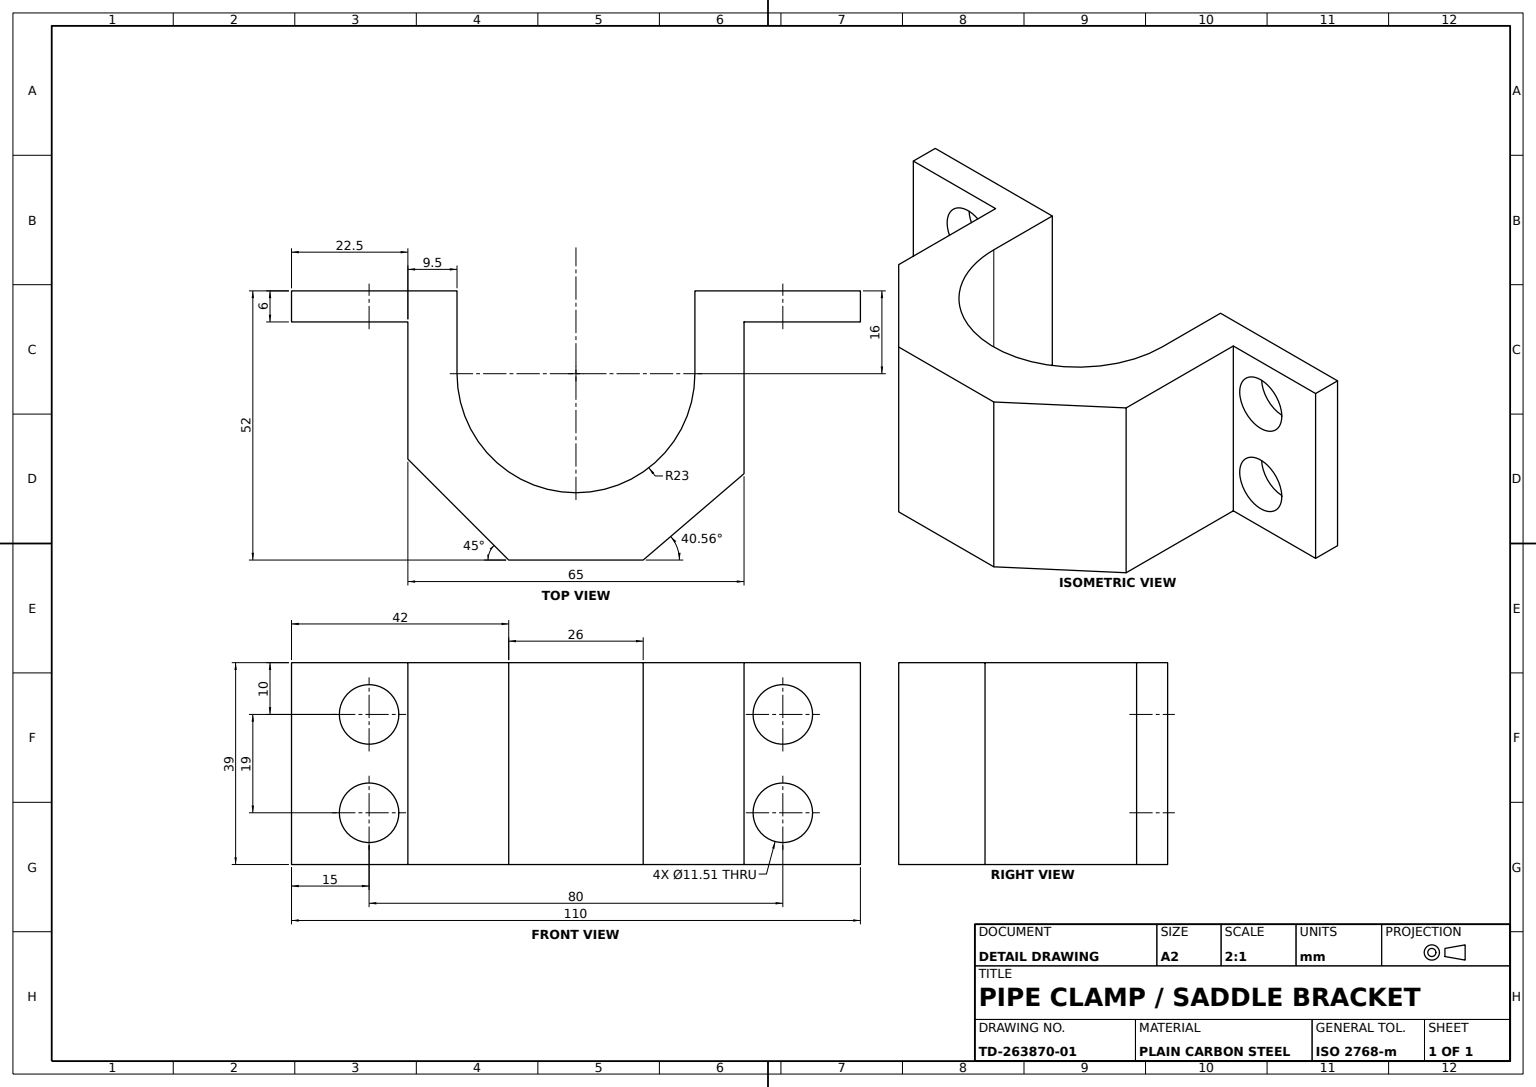
SolidWorks part; units mm, degrees
material "Plain Carbon Steel"
ref_plane "Front Plane" through (0, 0, 0) normal (0, 0, 1) x (1, 0, 0)
ref_plane "Top Plane" through (0, 0, 0) normal (0, 1, 0) x (1, 0, 0)
ref_plane "Right Plane" through (0, 0, 0) normal (1, 0, 0) x (0, 0, -1)
sketch "Saddle Profile Sketch" plane through (0, 0, 0) normal (0, 1, 0) x (1, 0, 0)
  line L0 (-23, -0.3099) -> (-23, -16.3099)
  line L1 (-55, -0.3099) -> (-23, -0.3099)
  line L2 (-55, -0.3099) -> (-55, -6.3099)
  line L3 (-55, -6.3099) -> (-32.5, -6.3099)
  line L4 (55, -0.3099) -> (55, -6.3099)
  line L7 (23, -0.3099) -> (23, -16.3099)
  line L8 (23, -0.3099) -> (55, -0.3099)
  line L11 (32.5, -6.3099) -> (55, -6.3099)
  line L12 (-32.5, -6.3099) -> (-32.5, -32.8099)
  line L13 (-32.5, -32.8099) -> (-13, -52.3099)
  line L14 (-13, -52.3099) -> (13, -52.3099)
  line L15 (13, -52.3099) -> (32.5, -35.6193)
  line L16 (32.5, -35.6193) -> (32.5, -6.3099)
  line L17 (0, 0) -> (0, -71.0885) construction
  arc A1 (-23, -16.3099) -> (23, -16.3099) centre (0, -16.3099) ccw
  point P0 (0, 0)
  dimension "D4" = 26
  dimension "D11" = 23
  dimension "D1" = 6
  dimension "D2" = 110
  dimension "D3" = 16
  dimension "D5" = 13
  dimension "D6" = 45
  dimension "D7" = 40.561
  dimension "D8" = 65
  dimension "D9" = 32.5
  dimension "D10" = 52
  dimension "D12" = 22.5
  dimension "D13" = 52.3099
extrude "Saddle Body" add sketch "Saddle Profile Sketch" along normal mid plane 39
sketch "Flange Holes Sketch" plane through (0, 0, 0.3099) normal (0, 0, -1) x (-1, 0, 0)
  circle A0 centre (-40, 9.5) radius 5.7548
  circle A1 centre (40, 9.5) radius 5.7548
  circle A2 centre (40, -9.5) radius 5.7548
  circle A3 centre (-40, -9.5) radius 5.7548
  dimension "D3" = 40
  dimension "D7" = 11.5095
  dimension "D1" = 80
  dimension "D2" = 80
  dimension "D4" = 40
  dimension "D5" = 19
  dimension "D6" = 9.5
extrude "Flange Bolt Holes" cut sketch "Flange Holes Sketch" against normal blind 39
